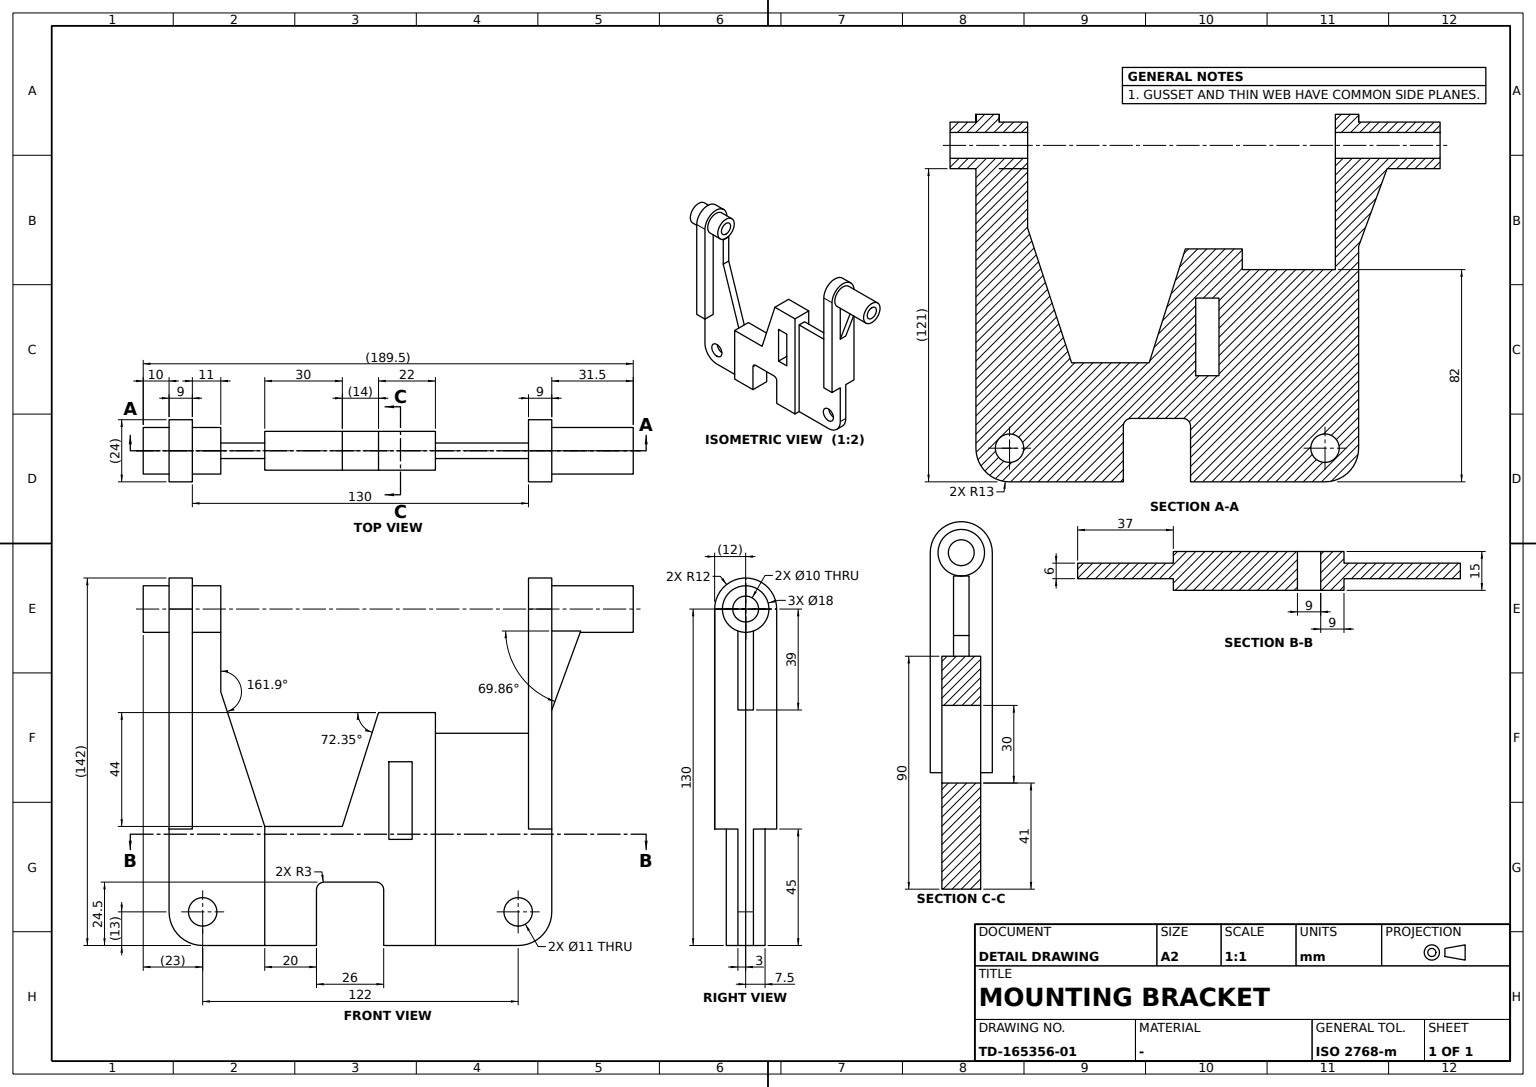
CATIA V5 part; units mm, degrees
sketch "Sketch1" plane through (0, 0, 0) normal (1, 0, 0) x (0, 1, 0)
  point P0 (-33, 46)
  line L0 (-33, 46) -> (-33, 0)
  point P1 (-33, 0)
  line L1 (-33, 0) -> (-13, 0)
  line L2 (-13, 0) -> (-13, 21.5)
  point P2 (-13, 24.5)
  line L3 (-10, 24.5) -> (10, 24.5)
  point P3 (13, 24.5)
  line L4 (13, 21.5) -> (13, 0)
  point P4 (13, 0)
  line L5 (13, 0) -> (33, 0)
  line L6 (33, 0) -> (33, 90)
  line L7 (33, 90) -> (11, 90)
  line L8 (11, 90) -> (-3, 46)
  line L9 (-3, 46) -> (-33, 46)
  point P5 (-33, 46)
  arc A0 (13, 21.5) -> (10, 24.5) centre (10, 21.5) ccw
  line L10 (15, 71) -> (24, 71)
  line L11 (24, 71) -> (24, 41)
  line L12 (24, 41) -> (15, 41)
  line L13 (15, 41) -> (15, 71)
  arc A1 (-13, 21.5) -> (-10, 24.5) centre (-10, 21.5) cw
  dimension "length L5" = 20
  dimension "length L1" = 20
  dimension "length L6" = 90
  dimension "length L9" = 30
  dimension "distance L7 L9" = 44
  dimension "length L7" = 22
  dimension "distance P3 P4" = 24.5
  dimension "distance P2 P3" = 26
  dimension "radius A0" = 3
  dimension "length L11" = 30
  dimension "distance L12 L5" = 41
  dimension "length L12" = 9
  dimension "distance L11 L6" = 9
  dimension "radius A1" = 3
  constraint coincidence P1 x-axis
  constraint coincidence P4 x-axis
  constraint coincidence P5 L0
  constraint coincidence P0 P5
  constraint coincidence L4 P3
  constraint coincidence L3 P3
  constraint coincidence L2 P2
  constraint coincidence L3 P2
  constraint vertical L0 y-axis
  constraint vertical L2 y-axis
  constraint vertical L4 y-axis
  constraint vertical L6 y-axis
  constraint vertical L11 y-axis
  constraint vertical L13 y-axis
  constraint horizontal L1 x-axis
  constraint horizontal L3 x-axis
  constraint horizontal L5 x-axis
  constraint horizontal L7 x-axis
  constraint horizontal L9 x-axis
  constraint horizontal L10 x-axis
  constraint horizontal L12 x-axis
  constraint symmetry L0 L6 y-axis
  constraint tangency A0 L4
  constraint tangency A0 L3
  constraint tangency A1 L2
  constraint tangency A1 L3
extrude "Pad1" add sketch "Sketch1" along normal mid plane 15
sketch "Sketch2" plane through (0, 0, 0) normal (1, 0, 0) x (0, 1, 0)
  line L0 (33, 0) -> (33, 90) construction
  line L1 (33, 0) -> (33, 82)
  point P0 (33, 0)
  line L2 (33, 0) -> (65, 0)
  point P1 (78, 0)
  line L3 (78, 13) -> (78, 45)
  point P2 (78, 45)
  line L4 (78, 45) -> (69, 45)
  line L5 (69, 45) -> (69, 82)
  line L6 (69, 82) -> (33, 82)
  point P3 (33, 82)
  arc A0 (65, 0) -> (78, 13) centre (65, 13) ccw
  circle A1 centre (65, 13) radius 5.5
  dimension "length L4" = 9
  dimension "distance L6 L2" = 82
  dimension "distance P0 P1" = 45
  dimension "distance P1 P2" = 45
  dimension "radius A0" = 13
  dimension "radius A1" = 5.5
  constraint horizontal L2 x-axis
  constraint horizontal L4 x-axis
  constraint horizontal L6 x-axis
  constraint vertical L3 y-axis
  constraint vertical L5 y-axis
  constraint coincidence P3 L0
  constraint coincidence L2 P1
  constraint coincidence L3 P1
  constraint tangency A0 L2
  constraint tangency A0 L3
extrude "Pad2" add sketch "Sketch2" along normal mid plane 6
sketch "Sketch3" plane through (0, 0, 0) normal (1, 0, 0) x (0, 1, 0)
  line L0 (-33, 46) -> (-33, 0)
  point P0 (-33, 0)
  line L1 (-33, 0) -> (-57, 0)
  point P1 (-70, 0)
  line L2 (-70, 13) -> (-70, 45)
  point P2 (-70, 45)
  line L3 (-70, 45) -> (-61, 45)
  line L4 (-61, 45) -> (-61, 121)
  line L5 (-61, 121) -> (-50, 121)
  line L6 (-50, 121) -> (-50, 98)
  line L7 (-50, 98) -> (-33, 46)
  arc A0 (-70, 13) -> (-57, 0) centre (-57, 13) ccw
  circle A1 centre (-57, 13) radius 5.5
  dimension "length L3" = 9
  dimension "length L5" = 11
  dimension "length L6" = 23
  dimension "distance L1 L5" = 121
  dimension "distance P1 P2" = 45
  dimension "distance P0 P1" = 37
  dimension "radius A0" = 13
  dimension "radius A1" = 5.5
  constraint horizontal L1 x-axis
  constraint horizontal L3 x-axis
  constraint horizontal L5 x-axis
  constraint vertical L2 y-axis
  constraint vertical L4 y-axis
  constraint vertical L6 y-axis
  constraint coincidence L2 P1
  constraint coincidence L1 P1
  constraint tangency A0 L2
  constraint tangency A0 L1
extrude "Pad3" add sketch "Sketch3" along normal mid plane 6
sketch "Sketch4" plane through (0, 69, 0) normal (0, 1, 0) x (-1, 0, 0)
  line L0 (3, 45) -> (-3, 45)
  line L1 (3, 45) -> (12, 45)
  line L2 (12, 45) -> (12, 130)
  arc A0 (12, 130) -> (-12, 130) centre (0, 130) ccw
  point P0 (0, 130)
  line L3 (-12, 130) -> (-12, 45)
  point P1 (-12, 45)
  line L4 (-12, 45) -> (-3, 45)
  dimension "radius A0" = 12
  dimension "distance P0 x axis" = 130
  constraint horizontal L1 x-axis
  constraint horizontal L4 x-axis
  constraint vertical L2 y-axis
  constraint tangency A0 L2
  constraint tangency L3 A0
  constraint coincidence P1 L0
  constraint symmetry L3 L2 y-axis
extrude "Pad4" add sketch "Sketch4" along normal blind 9
sketch "Sketch5" plane through (0, 78, 0) normal (0, 1, 0) x (-1, 0, 0)
  circle A0 centre (0, 130) radius 9
  point P0 (0, 130)
  circle A1 centre (0, 130) radius 5
  dimension "radius A0" = 9
  dimension "radius A1" = 5
  dimension "distance P0 x axis" = 130
  constraint coincidence P0 y-axis
extrude "Pad5" add sketch "Sketch5" along normal blind 31.5
sketch "Sketch6" plane through (0, 0, 0) normal (1, 0, 0) x (0, 1, 0)
  line L0 (89, 121) -> (78, 91)
  point P0 (89, 121)
  point P1 (78, 91)
  line L1 (78, 45) -> (78, 13) construction
  line L2 (78, 130) -> (78, 45) construction
  dimension "D1" = 9
  dimension "distance P0 L2" = 11
  dimension "distance P1 P0 y axis" = 30
  constraint coincidence L1 P1
rib "Stiffener1" sketch "Sketch6" thickness 6 sides both
sketch "Sketch7" plane through (0, -61, 0) normal (0, -1, 0) x (1, 0, 0)
  line L0 (-1.4609, 45) -> (12, 45)
  line L1 (12, 45) -> (12, 130)
  arc A0 (12, 130) -> (-12, 130) centre (0, 130) ccw
  point P0 (0, 130)
  line L2 (-12, 130) -> (-12, 45)
  point P1 (-12, 45)
  line L3 (-12, 45) -> (-1.4609, 45)
  dimension "radius A0" = 12
  dimension "distance P0 x axis" = 130
  dimension "distance L0 x axis" = 45
  constraint horizontal L0 x-axis
  constraint horizontal L3 x-axis
  constraint vertical L1 y-axis
  constraint tangency A0 L1
  constraint tangency L2 A0
  constraint coincidence P1 L0
  constraint symmetry L2 L1 y-axis
extrude "Pad6" add sketch "Sketch7" along normal blind 9
sketch "Sketch8" plane through (0, -70, 0) normal (0, -1, 0) x (1, 0, 0)
  circle A0 centre (0, 130) radius 9
  point P0 (0, 130)
  dimension "radius A0" = 9
  dimension "distance P0 x axis" = 130
  constraint coincidence P0 y-axis
extrude "Pad7" add sketch "Sketch8" along normal blind 10
sketch "Sketch9" plane through (0, -61, 0) normal (0, 1, 0) x (-1, 0, 0)
  circle A0 centre (0, 130) radius 9
extrude "Pad8" add sketch "Sketch9" along normal blind 11
sketch "Sketch10" plane through (0, -80, 0) normal (0, -1, 0) x (1, 0, 0)
  circle A0 centre (0, 130) radius 5
  point P0 (0, 130)
  circle A1 centre (0, 130) radius 9 construction
  dimension "radius A0" = 5
  constraint coincidence P0 y-axis
  constraint concentricity A0 A1
extrude "Pocket1" cut sketch "Sketch10" against normal through all
properties part number "bracket"
